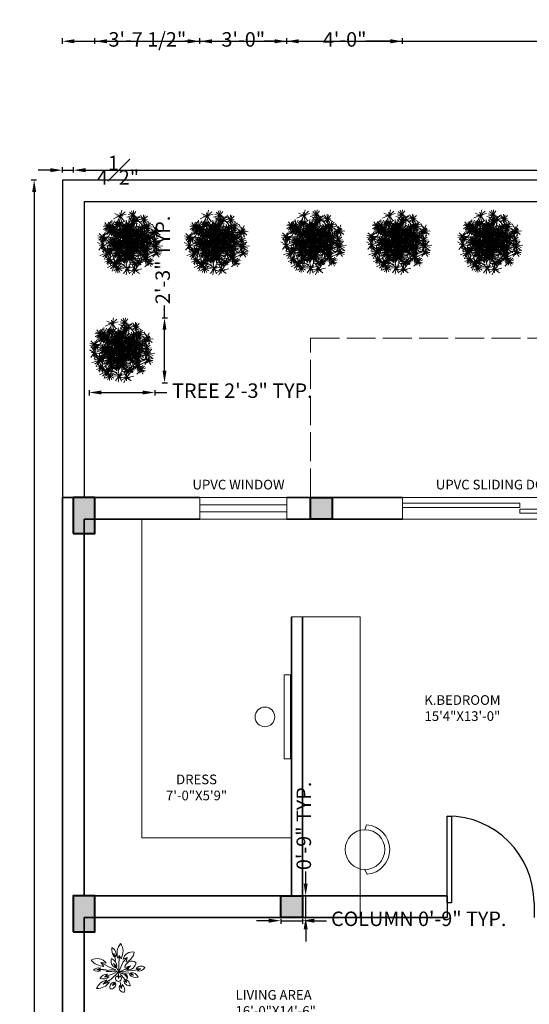
# Model space of a CAD drawing. Units: inches. Extents: x 2845 to 3575, y 808 to 1996.
# Tile 5 of 6: x 2955 to 3166, y 1588 to 1996. Entities that reach past the tile are written whole.
import ezdxf

# ---------------------------------------------------------------- set-up
doc = ezdxf.new("R2010")
doc.units = ezdxf.units.IN
doc.linetypes.add('ACAD_ISO02W100', pattern=[15, 12, -3])
for name, color, linetype, lineweight in [('A-ANNO-DIMS', 2, 'Continuous', 18), ('A-ANNO-TEXT', 7, 'Continuous', 18), ('A-AREA-IDEN', 7, 'Continuous', 18), ('A-COLS', 7, 'Continuous', 40), ('A-COLS-PATT', 212, 'Continuous', 13), ('A-DOOR', 34, 'Continuous', 25), ('A-FLOR-CASE', 30, 'Continuous', 18), ('A-FURN', 30, 'Continuous', 18), ('A-GLAZ', 4, 'Continuous', 18), ('A-ROOF-OVHD', 7, 'ACAD_ISO02W100', 18), ('A-WALL', 1, 'Continuous', 35), ('C-PROP', 7, 'Continuous', 30), ('L-PLNT', 3, 'Continuous', 13)]:
    doc.layers.add(name, color=color, linetype=linetype, lineweight=lineweight)
doc.styles.get("Standard").update_dxf_attribs({"font": 'arial.ttf'})
doc.dimstyles.new('ISO-25', dxfattribs={"dimtxt": 6, "dimasz": 5, "dimexe": 1.25, "dimexo": 0.625, "dimtad": 0, "dimlunit": 4, "dimtxsty": 'Standard', "dimcen": 2.5, "dimclrd": 1, "dimclre": 1, "dimclrt": 1, "dimadec": 0, "dimazin": 0, "dimtfac": 1, "dimtmove": 0, "dimatfit": 3, "dimfxl": 1, "dimfxlon": 1, "dimfrac": 1, "dimarcsym": 0})

# ---------------------------------------------------------------- blocks, each defined once
blk = doc.blocks.new('*U3')
for p, q in [((0, 0), (0, -6)), ((36, 0), (36, -6))]:
    blk.add_line(p, q)
blk.add_lwpolyline([(0, 0), (0, 36), (1.75, 36), (1.75, 0)], close=True)
blk.add_arc((0, 0), 36, 0, 90)
blk = doc.blocks.new('z_96')
for p, q in [((-282, 143), (-440, 264)), ((-279, 140), (-327, 271)), ((-280, 150), (-254, 304)), ((-277, 144), (-209, 319)), ((2, 182), (-93, 262)), ((-2, 184), (-55, 292)), ((1, 182), (29, 300)), ((4, 189), (59, 265)), ((6, 185), (92, 285)), ((-283, 139), (-471, 115)), ((-292, 134), (-431, 180)), ((-279, 142), (-398, 17)), ((-286, 137), (-375, 92)), ((-278, 140), (-313, -1)), ((-279, 135), (-307, 100)), ((-280, 150), (-304, 174)), ((-278, 131), (-222, 40)), ((-277, 137), (-129, 19)), ((-276, 141), (-147, 221)), ((-18, -6), (-275, 142)), ((-263, 140), (-131, 114)), ((-260, 142), (-98, 156)), ((-10, 183), (-130, 223)), ((-75, -25), (-112, 38)), ((-6, 186), (-100, 114)), ((-5, 182), (-87, 72)), ((-72, -35), (-42, 65)), ((-5, -3), (1, 176)), ((-1, 185), (126, 194)), ((0, 0), (389, 84)), ((2, 183), (70, 78)), ((10, 182), (88, 115)), ((164, -90), (143, 12)), ((163, -89), (239, 8)), ((393, 90), (274, 50)), ((393, 90), (285, 153)), ((393, 90), (294, 12)), ((393, 90), (354, 209)), ((391, 83), (363, 42)), ((393, 90), (479, 182)), ((393, 90), (515, 124)), ((393, 90), (494, 13)), ((393, 90), (517, 64)), ((393, 90), (443, -26)), ((396, 95), (439, 246)), ((409, 93), (456, 89)), ((-237, -199), (-392, -169)), ((-242, -196), (-391, -241)), ((-242, -199), (-330, -310)), ((-246, -194), (-283, -164)), ((-237, -199), (-267, -22)), ((-241, -202), (-259, -277)), ((-242, -202), (-48, -207)), ((-10, -6), (-236, -205)), ((-236, -201), (-139, -307)), ((-234, -202), (-196, -41)), ((-231, -196), (-205, -162)), ((-231, -206), (-147, -236)), ((-75, -39), (-157, -75)), ((-74, -33), (-152, -41)), ((-65, -33), (-136, -11)), ((-76, -36), (-103, -106)), ((-80, -29), (-90, -20)), ((-16, -6), (-75, -37)), ((-73, -35), (-72, -112)), ((-70, -40), (-38, -103)), ((-70, -41), (4, -57)), ((-68, -28), (-56, -19)), ((-5, -19), (164, -92)), ((167, -95), (37, -175)), ((161, -92), (74, -95)), ((159, -86), (86, -29)), ((164, -102), (119, -171)), ((163, -86), (138, -56)), ((164, -93), (157, -141)), ((160, -93), (268, -148)), ((164, -92), (234, -170)), ((165, -92), (296, -74)), ((167, -88), (276, -25)), ((167, -91), (187, -100)), ((167, -104), (188, -213)), ((168, -88), (194, -72))]:
    blk.add_line(p, q)
blk = doc.blocks.new('сосна 1')
for p, rotation in [((-413, 387), 205.4822314301707), ((318, 388), 121.1570021628385), ((-343, -102), 57.88453704712605), ((-351, 122), 257.3134436407499), ((-143, -5), 121.1570021628385), ((-137, 361), 177.7388340989747), ((-117, 122), 55.05972244949475), ((286, 9), 60.73020616460848), ((234, -65), 73.8676290404427), ((-274, 161), 177.7388340989747), ((98, -5), 177.7388340989747), ((174, 17), 349.7944254651076), ((327, 46), 177.7388340989747), ((-502, -282), 279.7984529833926), ((-175, -367), 63.19571700542104), ((-49, -394), 342.5348703671633), ((261, -459), 13.72293452966709)]:
    blk.add_blockref('z_96', p, dxfattribs=dict(rotation=rotation))
blk = doc.blocks.new('z_109')
for p, q in [((-392, 202), (-278, 190)), ((-254, 128), (-392, 202)), ((-94, 294), (-122, 396)), ((-121, 393), (-119, 324)), ((-120, 377), (-82, 322)), ((-85, 244), (-94, 293)), ((-5, 350), (-42, 295)), ((-20, 11), (-18, 230)), ((-20, 11), (65, 205)), ((-14, 234), (-5, 350)), ((-5, 350), (24, 284)), ((65, 209), (150, 307)), ((65, 205), (65, 205)), ((150, 307), (68, 272)), ((129, 216), (150, 307)), ((150, 307), (129, 216)), ((-342, 60), (-472, 63)), ((-467, 63), (-392, 90)), ((-463, 64), (-392, 37)), ((-390, 202), (-327, 125)), ((-276, 53), (-338, 57)), ((-84, 54), (-246, 125)), ((-20, 11), (-181, -143)), ((-61, 92), (-128, 186)), ((-126, 184), (-60, 125)), ((-120, 176), (-91, 98)), ((-20, 11), (-61, 92)), ((-20, 11), (-24, -65)), ((-20, 11), (102, 64)), ((-20, 11), (-14, 11)), ((-14, 11), (319, 50)), ((-14, 11), (-13, 13)), ((-13, 13), (13, -13)), ((217, 135), (101, 105)), ((102, 64), (217, 135)), ((217, 135), (145, 55)), ((319, 50), (434, 75)), ((429, 74), (333, 77)), ((428, 74), (353, 32)), ((-187, -143), (-345, -240)), ((-342, -238), (-269, -151)), ((-328, -230), (-213, -195)), ((-178, -41), (-313, -92)), ((-308, -90), (-254, -33)), ((-306, -89), (-217, -88)), ((-86, -8), (-178, -41)), ((-89, -192), (-150, -267)), ((-150, -266), (-131, -199)), ((-26, -113), (-45, -66)), ((-24, -65), (-28, -121)), ((-28, -117), (-2, -69)), ((4, -192), (16, -238)), ((16, -43), (88, -126)), ((141, -208), (84, -170)), ((87, -129), (140, -204)), ((122, -8), (193, -11)), ((140, -205), (123, -139)), ((176, -10), (285, -54)), ((283, -54), (196, -42)), ((273, -52), (222, -4)), ((-151, -267), (-81, -228)), ((34, -320), (-6, -268)), ((16, -238), (35, -326)), ((35, -327), (45, -249))]:
    blk.add_line(p, q)
for centre, radius, start, end in [((84, 468), 249, 170.3029, 215.3262), ((-235, 368), 160, 343.2534, 62.5239), ((262, 393), 319, 140.563, 197.8988), ((-221, 433), 288, 328.6458, 34.5329), ((256, 231), 192, 77.7318, 167.6805), ((55, 447), 242, 287.7269, 353.3689), ((-464, 59), 228, 35.1725, 122.5976), ((-304, 504), 380, 221.8384, 266.6027), ((-21, 239), 158, 161.4501, 243.415), ((-251, 115), 192, 2.9136, 65.0019), ((247, 86), 147, 55.2824, 172.6291), ((167, 217), 164, 262.2896, 356.2544), ((-434, -39), 136, 71.6414, 139.5892), ((-450, 225), 197, 243.5199, 287.2599), ((-173, -118), 175, 44.3837, 127.1057), ((-243, -1063), 1086, 79.6239, 91.8656), ((434, 8), 123, 51.1111, 145.9654), ((384, 175), 146, 257.8549, 330.7421), ((-198, -444), 302, 103.499, 156.8265), ((-455, -39), 287, 265.8156, 327.2626), ((-246, -222), 190, 92.4489, 147.0817), ((-337, 52), 185, 248.0932, 310.529), ((-94, -301), 109, 109.8936, 199.3062), ((-31, -123), 58.9, 103.4106, 268.148), ((-26, -123), 58.9, 262.5922, 66.6581), ((53, -110), 105, 354.7987, 111.9005), ((2, -181), 167, 21.6922, 85.2277), ((197, -160), 113, 185.1842, 278.9266), ((66, -276), 148, 1.4924, 67.3596), ((325, 60), 164, 218.6232, 288.4099), ((241, -149), 146, 21.4559, 97.3107), ((-186, -232), 105, 264.4232, 2.0221), ((80, -308), 95.1, 155.1092, 275.9038), ((-28, -354), 128, 337.3115, 55.0978)]:
    blk.add_arc(centre, radius, start, end)
blk = doc.blocks.new('*D22')
at = {"layer": 'A-ANNO-DIMS', "color": 0, "lineweight": -2, "transparency": 16777216}
for p, q in [((2967.62, 1933.77), (2962.62, 1933.77)), ((2972.62, 1932.77), (2972.62, 1935.02)), ((2972.62, 1933.77), (2977.22, 1933.77)), ((2977.22, 1932.77), (2977.22, 1935.02)), ((2982.22, 1933.77), (2987.22, 1933.77))]:
    blk.add_line(p, q, dxfattribs=at)
at = {"layer": 'A-ANNO-DIMS', "color": 0, "transparency": 16777216}
for points in [[(2967.62, 1934.61), (2967.62, 1932.94), (2972.62, 1933.77)], [(2982.22, 1934.61), (2982.22, 1932.94), (2977.22, 1933.77)]]:
    blk.add_solid(points, dxfattribs=at)
at = {"layer": 'Defpoints', "color": 0, "transparency": 16777216}
for p in [(2977.22, 1933.77), (2972.62, 1929.67), (2977.22, 1929.67)]:
    blk.add_point(p, dxfattribs=at)
at = {"layer": 'A-ANNO-DIMS', "color": 0, "transparency": 16777216, "insert": (2995.7, 1933.77), "char_height": 6, "attachment_point": 5}
blk.add_mtext('4{\\H1x;\\S1#2;}"', dxfattribs=at)
blk = doc.blocks.new('*D23')
at = {"layer": 'A-ANNO-DIMS', "color": 0, "lineweight": -2, "transparency": 16777216}
for p, q in [((2977.22, 1932.77), (2977.22, 1935.02)), ((2982.22, 1933.77), (3231.61, 1933.77)), ((3503.12, 1933.77), (3253.72, 1933.77)), ((3508.12, 1932.77), (3508.12, 1935.02))]:
    blk.add_line(p, q, dxfattribs=at)
at = {"layer": 'A-ANNO-DIMS', "color": 0, "transparency": 16777216}
for points in [[(2982.22, 1934.61), (2982.22, 1932.94), (2977.22, 1933.77)], [(3503.12, 1934.61), (3503.12, 1932.94), (3508.12, 1933.77)]]:
    blk.add_solid(points, dxfattribs=at)
at = {"layer": 'Defpoints', "color": 0, "transparency": 16777216}
for p in [(3508.12, 1933.77), (2977.22, 1929.67), (3508.12, 1920.75)]:
    blk.add_point(p, dxfattribs=at)
at = {"layer": 'A-ANNO-DIMS', "color": 0, "transparency": 16777216, "insert": (3242.67, 1933.77), "char_height": 6, "attachment_point": 5}
blk.add_mtext('44\'-3"', dxfattribs=at)
blk = doc.blocks.new('*D30')
at = {"layer": 'A-ANNO-DIMS', "color": 0, "lineweight": -2, "transparency": 16777216}
for p, q in [((2961.94, 1929.67), (2959.69, 1929.67)), ((2960.94, 1924.67), (2960.94, 1473.45)), ((2960.94, 987.17), (2960.94, 1438.39)), ((2961.94, 982.17), (2959.69, 982.17))]:
    blk.add_line(p, q, dxfattribs=at)
at = {"layer": 'A-ANNO-DIMS', "color": 0, "transparency": 16777216}
for points in [[(2960.11, 1924.67), (2961.77, 1924.67), (2960.94, 1929.67)], [(2960.11, 987.17), (2961.77, 987.17), (2960.94, 982.17)]]:
    blk.add_solid(points, dxfattribs=at)
at = {"layer": 'Defpoints', "color": 0, "transparency": 16777216}
for p in [(2972.62, 1929.67), (2960.94, 982.17), (2972.62, 982.17)]:
    blk.add_point(p, dxfattribs=at)
at = {"layer": 'A-ANNO-DIMS', "color": 0, "transparency": 16777216, "insert": (2960.94, 1455.92), "char_height": 6, "attachment_point": 5, "rotation": 90}
blk.add_mtext('78\'-11{\\H1x;\\S1#2;}"', dxfattribs=at)
blk = doc.blocks.new('COL-9x15')
h = blk.add_hatch(color=256)
h.dxf.hatch_style = 1
h.paths.add_polyline_path([(0, 0), (9, 0), (9, 15), (0, 15)])
blk.add_lwpolyline([(0, 0), (9, 0), (9, 15), (0, 15)], close=True)
blk = doc.blocks.new('COL-9x9')
h = blk.add_hatch(color=256)
h.dxf.hatch_style = 1
h.paths.add_polyline_path([(9, 9), (0, 9), (0, 0), (9, 0)])
blk.add_lwpolyline([(0, 9), (9, 9), (9, 0), (0, 0)], close=True)
blk = doc.blocks.new('GLAZ-SLIDER-97')
for p, q in [((0, 9), (0, 0)), ((0, 9), (97.12, 9)), ((97.12, 9), (97.12, 0)), ((0, 6.63), (48.56, 6.63)), ((48.56, 4.89), (0, 4.89)), ((48.56, 6.63), (48.56, 4.89)), ((48.56, 2.45), (48.56, 4.19)), ((48.56, 4.19), (97.12, 4.19)), ((0, 0), (97.12, 0)), ((97.12, 2.45), (48.56, 2.45))]:
    blk.add_line(p, q)
blk = doc.blocks.new('*D38')
at = {"layer": 'A-ANNO-DIMS', "color": 1, "lineweight": -2, "transparency": 16777216}
for p, q in [((2983.8, 1842.65), (2983.8, 1840.4)), ((2988.8, 1841.65), (3005.9, 1841.65)), ((3010.9, 1842.65), (3010.9, 1840.4)), ((3010.9, 1841.65), (3015.9, 1841.65))]:
    blk.add_line(p, q, dxfattribs=at)
at = {"layer": 'A-ANNO-DIMS', "color": 1, "transparency": 16777216}
for points in [[(2988.8, 1842.49), (2988.8, 1840.82), (2983.8, 1841.65)], [(3005.9, 1842.49), (3005.9, 1840.82), (3010.9, 1841.65)]]:
    blk.add_solid(points, dxfattribs=at)
at = {"layer": 'Defpoints', "color": 0, "transparency": 16777216}
for p in [(2983.8, 1845.72), (3010.9, 1845.72), (3010.9, 1841.65)]:
    blk.add_point(p, dxfattribs=at)
at = {"layer": 'A-ANNO-DIMS', "color": 1, "transparency": 16777216, "insert": (3047.23, 1841.65), "char_height": 6, "attachment_point": 5}
blk.add_mtext('TREE 2\'-3" TYP.', dxfattribs=at)
blk = doc.blocks.new('*D39')
at = {"layer": 'A-ANNO-DIMS', "color": 1, "lineweight": -2, "transparency": 16777216}
for p, q in [((3014.97, 1872.64), (3014.97, 1877.64)), ((3013.97, 1872.64), (3016.22, 1872.64)), ((3014.97, 1850.72), (3014.97, 1867.64)), ((3013.97, 1845.72), (3016.22, 1845.72))]:
    blk.add_line(p, q, dxfattribs=at)
at = {"layer": 'A-ANNO-DIMS', "color": 1, "transparency": 16777216}
for points in [[(3014.14, 1867.64), (3015.8, 1867.64), (3014.97, 1872.64)], [(3014.14, 1850.72), (3015.8, 1850.72), (3014.97, 1845.72)]]:
    blk.add_solid(points, dxfattribs=at)
at = {"layer": 'Defpoints', "color": 0, "transparency": 16777216}
for p in [(3010.9, 1872.64), (3014.97, 1872.64), (3010.9, 1845.72)]:
    blk.add_point(p, dxfattribs=at)
at = {"layer": 'A-ANNO-DIMS', "color": 1, "transparency": 16777216, "insert": (3014.97, 1896.6), "char_height": 6, "attachment_point": 5, "rotation": 90}
blk.add_mtext('2\'-3" TYP.', dxfattribs=at)
blk = doc.blocks.new('*D46')
at = {"layer": 'A-ANNO-DIMS', "color": 1, "lineweight": -2, "transparency": 16777216}
for p, q in [((3058.12, 1622.82), (3053.12, 1622.82)), ((3063.12, 1623.55), (3063.12, 1621.57)), ((3063.12, 1622.82), (3072.12, 1622.82)), ((3072.12, 1623.55), (3072.12, 1621.57)), ((3077.12, 1622.82), (3082.12, 1622.82))]:
    blk.add_line(p, q, dxfattribs=at)
at = {"layer": 'A-ANNO-DIMS', "color": 1, "transparency": 16777216}
for points in [[(3058.12, 1623.66), (3058.12, 1621.99), (3063.12, 1622.82)], [(3077.12, 1623.66), (3077.12, 1621.99), (3072.12, 1622.82)]]:
    blk.add_solid(points, dxfattribs=at)
at = {"layer": 'Defpoints', "color": 0, "transparency": 16777216}
for p in [(3063.12, 1624.17), (3072.12, 1624.17), (3072.12, 1622.82)]:
    blk.add_point(p, dxfattribs=at)
at = {"layer": 'A-ANNO-DIMS', "color": 1, "transparency": 16777216, "insert": (3120.32, 1622.82), "char_height": 6, "attachment_point": 5}
blk.add_mtext('COLUMN 0\'-9" TYP.', dxfattribs=at)
blk = doc.blocks.new('*D47')
at = {"layer": 'A-ANNO-DIMS', "color": 1, "lineweight": -2, "transparency": 16777216}
for p, q in [((3073.47, 1638.17), (3073.47, 1643.17)), ((3072.74, 1633.17), (3074.72, 1633.17)), ((3073.47, 1624.17), (3073.47, 1633.17)), ((3072.74, 1624.17), (3074.72, 1624.17)), ((3073.47, 1619.17), (3073.47, 1614.17))]:
    blk.add_line(p, q, dxfattribs=at)
at = {"layer": 'A-ANNO-DIMS', "color": 1, "transparency": 16777216}
for points in [[(3072.63, 1638.17), (3074.3, 1638.17), (3073.47, 1633.17)], [(3072.63, 1619.17), (3074.3, 1619.17), (3073.47, 1624.17)]]:
    blk.add_solid(points, dxfattribs=at)
at = {"layer": 'Defpoints', "color": 0, "transparency": 16777216}
for p in [(3072.12, 1633.17), (3073.47, 1633.17), (3072.12, 1624.17)]:
    blk.add_point(p, dxfattribs=at)
at = {"layer": 'A-ANNO-DIMS', "color": 1, "transparency": 16777216, "insert": (3073.47, 1662.08), "char_height": 6, "attachment_point": 5, "rotation": 90}
blk.add_mtext('0\'-9" TYP.', dxfattribs=at)
blk = doc.blocks.new('*D70')
at = {"layer": 'A-ANNO-DIMS', "color": 1, "lineweight": -2, "transparency": 16777216}
for p, q in [((2972.62, 1986.17), (2972.62, 1988.42)), ((2977.62, 1987.17), (3231.56, 1987.17)), ((3507.62, 1987.17), (3253.67, 1987.17)), ((3512.62, 1986.17), (3512.62, 1988.42))]:
    blk.add_line(p, q, dxfattribs=at)
at = {"layer": 'A-ANNO-DIMS', "color": 1, "transparency": 16777216}
for points in [[(2977.62, 1988.01), (2977.62, 1986.34), (2972.62, 1987.17)], [(3507.62, 1988.01), (3507.62, 1986.34), (3512.62, 1987.17)]]:
    blk.add_solid(points, dxfattribs=at)
at = {"layer": 'Defpoints', "color": 0, "transparency": 16777216}
for p in [(3512.62, 1987.17), (2972.62, 1929.67), (3512.62, 1929.67)]:
    blk.add_point(p, dxfattribs=at)
at = {"layer": 'A-ANNO-DIMS', "color": 1, "transparency": 16777216, "insert": (3242.62, 1987.17), "char_height": 6, "attachment_point": 5}
blk.add_mtext('45\'-0"', dxfattribs=at)
blk = doc.blocks.new('*D74')
at = {"layer": 'A-ANNO-DIMS', "color": 1, "lineweight": -2, "transparency": 16777216}
for p, q in [((3029.62, 1986.17), (3029.62, 1988.42)), ((3034.62, 1987.17), (3039.02, 1987.17)), ((3060.62, 1987.17), (3056.21, 1987.17)), ((3065.62, 1986.17), (3065.62, 1988.42))]:
    blk.add_line(p, q, dxfattribs=at)
at = {"layer": 'A-ANNO-DIMS', "color": 1, "transparency": 16777216}
for points in [[(3034.62, 1988.01), (3034.62, 1986.34), (3029.62, 1987.17)], [(3060.62, 1988.01), (3060.62, 1986.34), (3065.62, 1987.17)]]:
    blk.add_solid(points, dxfattribs=at)
at = {"layer": 'Defpoints', "color": 0, "transparency": 16777216}
for p in [(3065.62, 1987.17), (3029.62, 1798.17), (3065.62, 1798.17)]:
    blk.add_point(p, dxfattribs=at)
at = {"layer": 'A-ANNO-DIMS', "color": 1, "transparency": 16777216, "insert": (3047.62, 1987.17), "char_height": 6, "attachment_point": 5}
blk.add_mtext('3\'-0"', dxfattribs=at)
blk = doc.blocks.new('*D78')
at = {"layer": 'A-ANNO-DIMS', "color": 1, "lineweight": -2, "transparency": 16777216}
for p, q in [((2986.12, 1986.17), (2986.12, 1988.42)), ((2991.12, 1987.17), (2992.28, 1987.17)), ((3024.62, 1987.17), (3023.45, 1987.17)), ((3029.62, 1986.17), (3029.62, 1988.42))]:
    blk.add_line(p, q, dxfattribs=at)
at = {"layer": 'A-ANNO-DIMS', "color": 1, "transparency": 16777216}
for points in [[(2991.12, 1988.01), (2991.12, 1986.34), (2986.12, 1987.17)], [(3024.62, 1988.01), (3024.62, 1986.34), (3029.62, 1987.17)]]:
    blk.add_solid(points, dxfattribs=at)
at = {"layer": 'Defpoints', "color": 0, "transparency": 16777216}
for p in [(3029.62, 1987.17), (2986.12, 1798.17), (3029.62, 1798.17)]:
    blk.add_point(p, dxfattribs=at)
at = {"layer": 'A-ANNO-DIMS', "color": 1, "transparency": 16777216, "insert": (3007.87, 1987.17), "char_height": 6, "attachment_point": 5}
blk.add_mtext('3\'-7 1/2"', dxfattribs=at)
blk = doc.blocks.new('*D79')
at = {"layer": 'A-ANNO-DIMS', "color": 1, "lineweight": -2, "transparency": 16777216}
for p, q in [((3065.62, 1986.17), (3065.62, 1988.42)), ((3070.62, 1987.17), (3080.9, 1987.17)), ((3108.62, 1987.17), (3098.34, 1987.17)), ((3113.62, 1986.17), (3113.62, 1988.42))]:
    blk.add_line(p, q, dxfattribs=at)
at = {"layer": 'A-ANNO-DIMS', "color": 1, "transparency": 16777216}
for points in [[(3070.62, 1988.01), (3070.62, 1986.34), (3065.62, 1987.17)], [(3108.62, 1988.01), (3108.62, 1986.34), (3113.62, 1987.17)]]:
    blk.add_solid(points, dxfattribs=at)
at = {"layer": 'Defpoints', "color": 0, "transparency": 16777216}
for p in [(3113.62, 1987.17), (3065.62, 1798.17), (3113.62, 1798.17)]:
    blk.add_point(p, dxfattribs=at)
at = {"layer": 'A-ANNO-DIMS', "color": 1, "transparency": 16777216, "insert": (3089.62, 1987.17), "char_height": 6, "attachment_point": 5}
blk.add_mtext('4\'-0"', dxfattribs=at)

msp = doc.modelspace()

# ---------------------------------------------------------------- hatches: boundary and pattern name
at = {"layer": 'A-COLS-PATT'}
h = msp.add_hatch(color=256, dxfattribs=at)
h.dxf.hatch_style = 1
h.paths.add_polyline_path([(3084.388, 1798.173), (3075.388, 1798.173), (3075.388, 1789.173), (3084.388, 1789.173)])

# ---------------------------------------------------------------- linework, layer by layer
at = {"layer": 'A-COLS'}
msp.add_lwpolyline([(3075.459, 1798.173), (3084.459, 1798.173), (3084.459, 1789.173), (3075.459, 1789.173)], close=True, dxfattribs=at)
at = {"layer": 'A-DOOR'}
msp.add_line((3132.116, 1633.173), (3132.116, 1624.173), dxfattribs=at)
at = {"layer": 'A-FLOR-CASE'}
for p, q in [((3005.616, 1789.173), (3005.616, 1657.173)), ((3067.616, 1748.677), (3096.116, 1748.677)), ((3096.116, 1633.173), (3096.116, 1748.677)), ((3067.616, 1657.173), (3005.616, 1657.173)), ((3096.116, 1633.173), (3096.116, 1624.173))]:
    msp.add_line(p, q, dxfattribs=at)
at = {"layer": 'A-FURN'}
for p, q in [((3098.046, 1660.496), (3098.664, 1662.506)), ((3098.046, 1644.039), (3098.887, 1642.01))]:
    msp.add_line(p, q, dxfattribs=at)
msp.add_lwpolyline([(3067.184, 1724.699), (3064.614, 1724.699), (3064.614, 1689.822), (3067.184, 1689.822)], close=True, dxfattribs=at)
for centre, radius in [((3056.573, 1707.26), 4.083), ((3098.046, 1652.267), 8.228)]:
    msp.add_circle(centre, radius, dxfattribs=at)
msp.add_arc((3098.046, 1652.267), 10.258, 274.62309, 86.5495, dxfattribs=at)
at = {"layer": 'A-GLAZ'}
for p, q in [((3029.616, 1798.173), (3029.616, 1789.173)), ((3029.616, 1798.173), (3065.616, 1798.173)), ((3029.616, 1795.173), (3065.616, 1795.173)), ((3065.616, 1798.173), (3065.616, 1789.173)), ((3029.616, 1792.173), (3065.616, 1792.173)), ((3029.616, 1789.173), (3065.616, 1789.173))]:
    msp.add_line(p, q, dxfattribs=at)
at = {"layer": 'A-ROOF-OVHD'}
for p, q in [((3075.459, 1798.173), (3075.459, 1864.202)), ((3075.459, 1864.202), (3263.616, 1864.202))]:
    msp.add_line(p, q, dxfattribs=at)
at = {"layer": 'A-WALL'}
for p, q in [((2972.616, 1798.173), (2972.616, 1143.734)), ((2981.616, 1798.173), (2972.616, 1798.173)), ((3029.616, 1798.173), (2981.616, 1798.173)), ((3113.616, 1798.173), (3065.616, 1798.173)), ((3029.616, 1789.173), (2981.616, 1789.173)), ((2981.616, 1789.173), (2981.616, 1633.173)), ((3113.616, 1789.173), (3065.616, 1789.173)), ((3067.616, 1633.173), (3067.616, 1748.677)), ((3072.116, 1633.173), (3072.116, 1748.677)), ((3132.116, 1633.173), (2981.616, 1633.173)), ((3132.116, 1624.173), (2981.616, 1624.173)), ((2981.616, 1624.173), (2981.616, 1450.173))]:
    msp.add_line(p, q, dxfattribs=at)
at = {"layer": 'C-PROP'}
for p, q in [((3512.616, 1929.673), (2972.616, 1929.673)), ((2972.616, 1929.673), (2972.616, 1798.173)), ((3503.616, 1920.673), (2981.616, 1920.673)), ((2981.616, 1920.673), (2981.616, 1798.173))]:
    msp.add_line(p, q, dxfattribs=at)

# ---------------------------------------------------------------- block references
at = {"layer": 'A-COLS'}
for name, p in [('COL-9x15', (2977.116, 1783.173)), ('COL-9x15', (2977.116, 1618.173)), ('COL-9x9', (3063.116, 1624.173))]:
    msp.add_blockref(name, p, dxfattribs=at)
at = {"layer": 'A-DOOR'}
msp.add_blockref('*U3', (3132.116, 1630.173), dxfattribs=at)
at = {"layer": 'A-GLAZ'}
msp.add_blockref('GLAZ-SLIDER-97', (3113.616, 1789.173), dxfattribs=at)
at = {"layer": 'L-PLNT'}
for name, p, xscale, yscale, zscale in [('сосна 1', (3001.291, 1903.918), 0.0163507860903289, 0.0163507860903289, 0.0163507860903289), ('сосна 1', (3037.256, 1903.917), 0.0163507860903289, 0.0163507860903289, 0.0163507860903289), ('сосна 1', (3077.354, 1904.174), 0.0163507860903289, 0.0163507860903289, 0.0163507860903289), ('сосна 1', (3112.746, 1904.174), 0.0163507860903289, 0.0163507860903289, 0.0163507860903289), ('сосна 1', (3150.523, 1904.174), 0.0163507860903289, 0.0163507860903289, 0.0163507860903289), ('сосна 1', (2997.934, 1859.423), 0.0163507860903289, 0.0163507860903289, 0.0163507860903289), ('z_109', (2996.437, 1601.346), 0.0202275909996564, 0.0202275909996564, 0.0202275909996564)]:
    msp.add_blockref(name, p, dxfattribs=dict(at, xscale=xscale, yscale=yscale, zscale=zscale))

# ---------------------------------------------------------------- texts
at = {"layer": 'A-ANNO-TEXT', "char_height": 4, "attachment_point": 1}
for s, width, insert in [('UPVC WINDOW', 45.255, (3026.548, 1805.497)), ('UPVC SLIDING DOOR', 60.26056, (3127.413, 1805.497))]:
    msp.add_mtext_dynamic_manual_height_columns(s, width=width, gutter_width=12.5, heights=[0], dxfattribs=dict(at, insert=insert))
at = {"layer": 'A-AREA-IDEN', "char_height": 4, "attachment_point": 1}
for s, insert in [('\\pxqc;K.BEDROOM\\P15\'4"X13\'-0"', (3115.798, 1716.247)), ('\\pxqc;DRESS\\P7\'-0"X5\'9"', (3005.616, 1683.342)), ('LIVING AREA\\P16\'-0"X14\'-6"', (3044.406, 1594.068))]:
    msp.add_mtext_dynamic_manual_height_columns(s, width=45.255, gutter_width=12.5, heights=[0], dxfattribs=dict(at, insert=insert))

# ---------------------------------------------------------------- dimensions: what is measured, and where the dimension line sits
at = {"layer": 'A-ANNO-DIMS'}
for base, p1, p2, override, picture, middle in [((3029.616, 1987.173), (2986.116, 1798.173), (3029.616, 1798.173), {"dimdec": 1, "dimlfac": 1, "dimrnd": 0, "dimzin": 1, "dimdsep": 46, "dimlunit": 4, "dimfrac": 2}, '*D78', (3007.866, 1987.173)), ((3512.616, 1987.173), (2972.616, 1929.673), (3512.616, 1929.673), {"dimdec": 1, "dimlfac": 1, "dimrnd": 0, "dimzin": 1, "dimdsep": 46, "dimlunit": 4, "dimfrac": 2}, '*D70', (3242.616, 1987.173)), ((3065.616, 1987.173), (3029.616, 1798.173), (3065.616, 1798.173), {"dimdec": 1, "dimlfac": 1, "dimrnd": 0, "dimzin": 1, "dimdsep": 46, "dimlunit": 4, "dimfrac": 2}, '*D74', (3047.616, 1987.173)), ((3113.616, 1987.173), (3065.616, 1798.173), (3113.616, 1798.173), {"dimdec": 1, "dimlfac": 1, "dimrnd": 0, "dimzin": 1, "dimdsep": 46, "dimlunit": 4, "dimfrac": 2}, '*D79', (3089.616, 1987.173)), ((2977.216, 1933.775), (2972.616, 1929.673), (2977.216, 1929.673), {"dimclrd": 0, "dimclre": 0, "dimclrt": 0}, '*D22', (2995.702, 1933.775)), ((3508.116, 1933.775), (2977.216, 1929.673), (3508.116, 1920.754), {"dimclrd": 0, "dimclre": 0, "dimclrt": 0, "dimtmove": 1}, '*D23', (3242.666, 1933.775))]:
    dim = msp.add_linear_dim(base=base, p1=p1, p2=p2, dimstyle='ISO-25', override=override, dxfattribs=at)
    dim.commit()
    dim.dimension.update_dxf_attribs({"geometry": picture, "text_midpoint": middle})
dim = msp.add_linear_dim(base=(2960.94, 982.173), p1=(2972.616, 1929.673), p2=(2972.616, 982.173), angle=90, dimstyle='ISO-25', override={"dimclrd": 0, "dimclre": 0, "dimclrt": 0}, dxfattribs=at)
dim.commit()
dim.dimension.update_dxf_attribs({"geometry": '*D30', "text_midpoint": (2960.94, 1455.923)})
for base, p1, p2, picture, middle in [((3014.97, 1872.641), (3010.904, 1845.717), (3010.904, 1872.641), '*D39', (3014.97, 1896.604)), ((3073.466, 1633.173), (3072.116, 1624.173), (3072.116, 1633.173), '*D47', (3073.466, 1662.084))]:
    dim = msp.add_linear_dim(base=base, p1=p1, p2=p2, angle=90, text='<> TYP.', dimstyle='ISO-25', override={"dimdec": 1, "dimlfac": 1, "dimrnd": 0, "dimzin": 1, "dimdsep": 46, "dimlunit": 4, "dimfrac": 2}, dxfattribs=at)
    dim.commit()
    dim.dimension.update_dxf_attribs({"geometry": picture, "text_midpoint": middle})
for base, p1, p2, text, picture, middle in [((3010.904, 1841.652), (2983.803, 1845.717), (3010.904, 1845.717), 'TREE <> TYP.', '*D38', (3047.233, 1841.652)), ((3072.116, 1622.823), (3063.116, 1624.173), (3072.116, 1624.173), 'COLUMN <> TYP.', '*D46', (3120.318, 1622.823))]:
    dim = msp.add_linear_dim(base=base, p1=p1, p2=p2, text=text, dimstyle='ISO-25', override={"dimdec": 1, "dimlfac": 1, "dimrnd": 0, "dimzin": 1, "dimdsep": 46, "dimlunit": 4, "dimfrac": 2}, dxfattribs=at)
    dim.commit()
    dim.dimension.update_dxf_attribs({"geometry": picture, "text_midpoint": middle})

doc.saveas('drawing.dxf')
